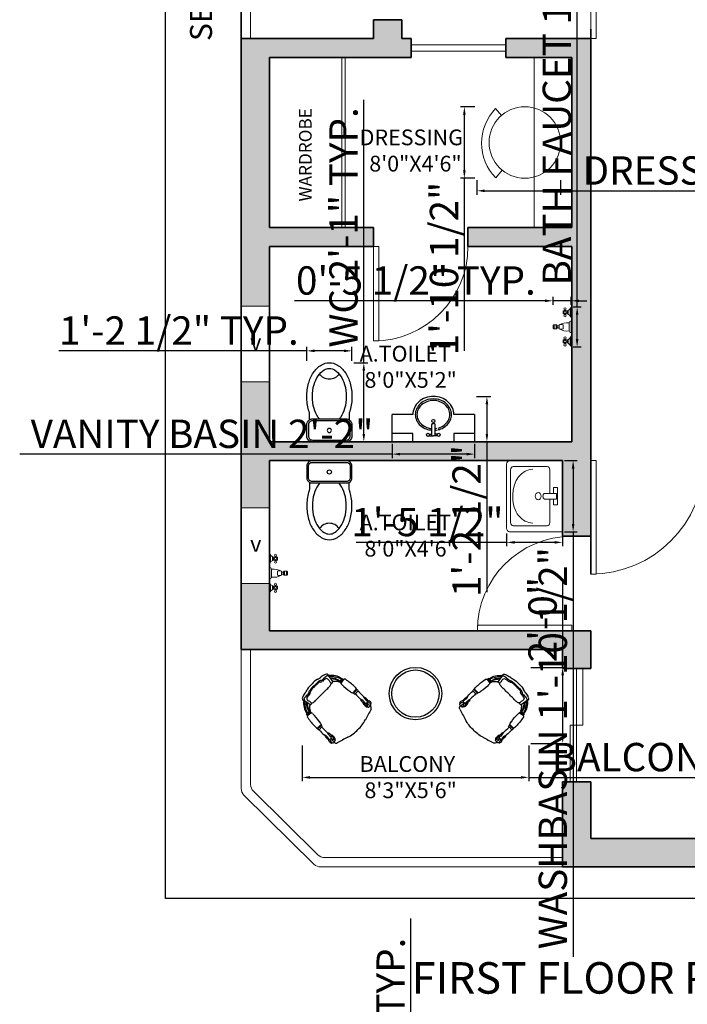
# Model space of a CAD drawing. Units: inches. Extents: x 3488 to 4319, y 780 to 1756.
# Tile 6 of 8: x 3844 to 4055, y 1274 to 1587. Entities that reach past the tile are written whole.
import ezdxf

# ---------------------------------------------------------------- set-up
doc = ezdxf.new("R2010")
doc.units = ezdxf.units.IN
for name, color, linetype, lineweight in [('A-ANNO-IDEN', 7, 'Continuous', 13), ('A-ANNO-TEXT', 7, 'Continuous', 18), ('A-ANNO-TITL', 7, 'Continuous', 25), ('A-AREA-IDEN', 7, 'Continuous', 18), ('A-DOOR', 4, 'Continuous', 18), ('A-FLOR-CASE', 32, 'Continuous', 18), ('A-FLOR-RAIL', 7, 'Continuous', 20), ('A-WALL', 7, 'Continuous', 35), ('A-WALL-PATT', 252, 'Continuous', 13), ('C-PROP', 7, 'Continuous', 25), ('DIM', 9, 'Continuous', 18), ('FUR', 42, 'Continuous', 18), ('window', 130, 'Continuous', 18), ('Сантехника', 9, 'Continuous', 18)]:
    doc.layers.add(name, color=color, linetype=linetype, lineweight=lineweight)
doc.layers.add('furn', color=7, linetype='Continuous')
doc.layers.add('SANTEH', color=7, linetype='Continuous')
doc.styles.get("Standard").update_dxf_attribs({"font": 'arial.ttf'})
doc.dimstyles.new('ISO-25', dxfattribs={"dimtxt": 9, "dimasz": 2.5, "dimexe": 1.25, "dimexo": 0.625, "dimtad": 1, "dimdec": 1, "dimlunit": 3, "dimtxsty": 'Standard', "dimcen": 2.5, "dimclrd": 1, "dimclre": 1, "dimclrt": 1, "dimadec": 0, "dimazin": 0, "dimtfac": 1, "dimtdec": 1, "dimtmove": 0, "dimatfit": 3, "dimfxl": 1, "dimarcsym": 0})

# ---------------------------------------------------------------- blocks, each defined once
blk = doc.blocks.new('*U3')
for p, q in [((0, 0), (0, -6)), ((36, 0), (36, -6))]:
    blk.add_line(p, q)
blk.add_lwpolyline([(0, 0), (0, 36), (1.75, 36), (1.75, 0)], close=True)
blk.add_arc((0, 0), 36, 0, 90)
blk = doc.blocks.new('*U9')
for p, q in [((0, 0), (0, 6)), ((36, 0), (36, 6))]:
    blk.add_line(p, q)
blk.add_lwpolyline([(0, 0), (0, -36), (1.75, -36), (1.75, 0)], close=True)
blk.add_arc((0, 0), 36, 270, 0)
blk = doc.blocks.new('*U10')
for p, q in [((0, 0), (0, 6)), ((30, 0), (30, 6))]:
    blk.add_line(p, q)
blk.add_lwpolyline([(0, 0), (0, -30), (1.75, -30), (1.75, 0)], close=True)
blk.add_arc((0, 0), 30, 270, 0)
blk = doc.blocks.new('*U11')
for p, q in [((-30, 0), (-30, 6)), ((0, 0), (0, 6))]:
    blk.add_line(p, q)
blk.add_lwpolyline([(0, 0), (0, -30), (-1.75, -30), (-1.75, 0)], close=True)
blk.add_arc((0, 0), 30, 180, 270)
blk = doc.blocks.new('K10-44')
at = {"layer": 'SANTEH'}
for points in [[(-182, 222.6, 0.020439), (-174, 197.6), (-174, 134.8, 0.262987), (-198.2, 92), (-198.2, -8, 0.414214), (-148.2, -58), (151.8, -58, 0.414214), (201.8, -8), (201.8, 92, 0.262987), (177.6, 134.8), (177.6, 197.6, 0.020439), (185.6, 222.6, 0.067459), (201.8, 342, 0.067459), (185.6, 461.3, 0.079812), (143.2, 554.1, 0.107118), (73.7, 621.5, 0.139889), (1.8, 642, 0.139889), (-70.1, 621.5, 0.107118), (-139.6, 554.1, 0.079812), (-182, 461.3, 0.067459), (-198.2, 342, 0.067459)], [(-148.2, 127), (151.8, 127, -0.414214), (186.8, 92), (186.8, -8, -0.414214), (151.8, -43), (-148.2, -43, -0.414214), (-183.2, -8), (-183.2, 92, -0.414214)]]:
    blk.add_lwpolyline(points, format="xyb", close=True, dxfattribs=at)
for points in [[(89.9, 142, 0.027307), (101.6, 157.6, 0.079812), (137.4, 235.9, 0.067459), (151.8, 342, 0.067459), (137.4, 448, 0.079812), (101.6, 526.4, 0.107118), (47.3, 579, 0.139889), (1.8, 592, 0.139889), (-43.7, 579, 0.107118), (-98, 526.4, 0.079812), (-133.8, 448, 0.067459), (-148.2, 342, 0.067459), (-133.8, 235.9, 0.079812), (-98, 157.6, 0.027307), (-86.4, 142, 0.139889)], [(-174, 134.8, -0.136371), (-148.2, 142), (151.8, 142, -0.136371), (177.6, 134.8)]]:
    blk.add_lwpolyline(points, format="xyb", dxfattribs=at)
blk.add_circle((1.8, 42), 18.3, dxfattribs=at)
blk.add_arc((1.8, 601.6), 105.3, 213.89944, 326.10056, dxfattribs=at)
blk = doc.blocks.new('s_20')
at = {"layer": 'SANTEH'}
for p, q in [((-1000, 0), (0, 0)), ((-1000, -330), (-1000, 0)), ((-750, -19), (-750, 0)), ((-250, 0), (-250, -100)), ((0, 0), (0, -330)), ((-1000, -100), (-750, -100)), ((-750, -100), (-750, -25)), ((-549, -73), (-500, -73)), ((-549, -93), (-520, -93)), ((-520, -73), (-520, -210)), ((-451, -73), (-500, -73)), ((-480, -73), (-480, -105)), ((-451, -93), (-480, -93)), ((-480, -109), (-480, -210)), ((-250, -100), (-35, -100)), ((-31, -100), (0, -100)), ((-510, -220), (-500, -220)), ((-490, -220), (-500, -220)), ((-1000, -330), (-750, -330)), ((-250, -330), (0, -330))]:
    blk.add_line(p, q, dxfattribs=at)
for points in [[(-720, -330, 0.110429), (-704, -400, 0.102661), (-657, -463, 0.093298), (-587, -505, 0.087608), (-500, -520, 0.087608), (-413, -505, 0.093298), (-343, -463, 0.102661), (-296, -400, 0.110429), (-280, -330, 0.110429), (-296, -260, 0.102661), (-343, -197, 0.093298), (-413, -155, 0.067743), (-480, -141, 0.087608)], [(-559, -147, 0.02908), (-587, -155, 0.093298), (-657, -197, 0.102661), (-704, -260, 0.110429), (-720, -330, 0.110429)], [(-700, -330, 0.110429), (-686, -391, 0.102661), (-644, -448, 0.093298), (-580, -486, 0.087608), (-500, -500, 0.087608), (-420, -486, 0.093298), (-356, -448, 0.102661), (-314, -391, 0.110429), (-300, -330, 0.110429), (-314, -269, 0.102661), (-356, -212, 0.093298), (-420, -174, 0.06604), (-480, -161, 0.087608)], [(-557, -167, 0.02562), (-580, -174, 0.093298), (-644, -212, 0.102661), (-686, -269, 0.110429), (-700, -330, 0.110429)], [(-520, -141, 0.028703), (-549, -145, 0.093298)], [(-520, -161, 0.024746), (-543, -164, 0.093298)], [(-750, -330, 0.110429), (-731, -413, 0.102661), (-677, -486, 0.093298), (-597, -533, 0.087608), (-500, -550, 0.087608), (-403, -533, 0.093298), (-323, -486, 0.102661), (-269, -413, 0.110429), (-250, -330, 0.110429)]]:
    blk.add_lwpolyline(points, format="xyb", dxfattribs=at)
for centre in [(-565, -84), (-435, -84), (-500, -252)]:
    blk.add_circle(centre, 18.9, dxfattribs=at)
for centre, start, end in [((-510, -210), 180, 270), ((-490, -210), 270, 0)]:
    blk.add_arc(centre, 10, start, end, dxfattribs=at)
blk = doc.blocks.new('Rac7')
at = {"color": 0}
for p, q in [((-39500.6, -24232.1), (-39500.6, -23829.6)), ((-39473.6, -23808.4), (-38988.3, -23808.4)), ((-39032.4, -23838), (-39429.6, -23838)), ((-38961.3, -23829.6), (-38961.3, -24232.1)), ((-39456.5, -23859.1), (-39456.5, -24114.9)), ((-39221.1, -23854.9), (-39240.8, -23854.9)), ((-39005.4, -24114.9), (-39005.4, -23859.1)), ((-39005.4, -23859.1), (-39005.4, -23859.1)), ((-39429.6, -24136.1), (-39252.5, -24136.1)), ((-39252.5, -24185.9), (-39252.5, -24093.6)), ((-39209.4, -24185.9), (-39209.4, -24093.6)), ((-39209.4, -24136.1), (-39032.4, -24136.1)), ((-39297, -24164), (-39252.5, -24164)), ((-39297, -24193.5), (-39297, -24164)), ((-39164.9, -24193.5), (-39297, -24193.5)), ((-39252.5, -24185.9), (-39209.4, -24185.9)), ((-39209.4, -24164), (-39164.9, -24164)), ((-39164.9, -24164), (-39164.9, -24193.5)), ((-38961.3, -24232.1), (-39500.6, -24232.1))]:
    blk.add_line(p, q, dxfattribs=at)
at = {"color": 0, "extrusion": (0, 0, -1)}
for centre, major_axis, start_param, end_param in [((-39473.6, -23829.6), (-27, 0), 0, 1.570796), ((-39429.6, -23859.1), (-27, 0), 0, 1.570796), ((-39032.4, -23859.1), (-27, 0), 1.570796, 3.141593), ((-38988.3, -23829.6), (-27, 0), 1.570796, 3.141593), ((-39240.8, -24007.4), (-194.1, 0), 0, 1.570796), ((-39221.1, -24007.4), (-194.1, 0), 1.570796, 3.141593), ((-39429.6, -24114.9), (-27, 0), -1.570796, 0), ((-39231, -24104), (-25.3, 0), 0.552816, 2.588777), ((-39032.4, -24114.9), (-27, 0), -3.141593, -1.570796)]:
    blk.add_ellipse(centre, major_axis=major_axis, ratio=0.785714, start_param=start_param, end_param=end_param, dxfattribs=at)
blk.add_ellipse((-39231, -24048), major_axis=(-27.9, 0), ratio=0.785714, dxfattribs=at)
blk = doc.blocks.new('Faucet - Bathroom front')
for p, q in [((-0.5, 4.25), (0.5, 4.25)), ((0.5, 3.75), (-0.5, 3.75)), ((-0.5, 3), (0.5, 3)), ((-0.25, 3), (-0.25, 3.5)), ((0.25, 3.5), (0.25, 3)), ((-5, 0), (-2.25, 0)), ((-4.5087, 0.25), (-2.7408, 0.25)), ((-4, 1.625), (-4.25, 1.625)), ((-4, 1.375), (-4.25, 1.375)), ((-3.1442, 0.75), (-4.0979, 0.75)), ((-3.25, 1.625), (-3, 1.625)), ((-3.25, 1.375), (-3, 1.375)), ((-1.5, 0), (1.5, 0)), ((-1, 0.5), (1, 0.5)), ((0.5, 2), (-0.5, 2)), ((2.25, 0), (5, 0)), ((2.7413, 0.25), (4.5092, 0.25)), ((3.25, 1.625), (3, 1.625)), ((3.25, 1.375), (3, 1.375)), ((4.1058, 0.75), (3.1521, 0.75)), ((4, 1.625), (4.25, 1.625)), ((4, 1.375), (4.25, 1.375))]:
    blk.add_line(p, q)
for points in [[(-0.5, 3.75), (-0.5, 4.25)], [(-0.25, 4.5), (0.25, 4.5)], [(0.25, 3.5), (-0.25, 3.5)], [(0.5, 4.25), (0.5, 3.75)]]:
    blk.add_lwpolyline(points)
for points in [[(-4, 1), (-4, 2), (-3.25, 2), (-3.25, 1)], [(3.25, 1), (3.25, 2), (4, 2), (4, 1)]]:
    blk.add_lwpolyline(points, close=True)
for centre in [(-4.5, 1.5), (-3.625, 1.5), (-2.75, 1.5), (2.75, 1.5), (3.625, 1.5), (4.5, 1.5)]:
    blk.add_circle(centre, 0.2795)
for centre, radius, start, end in [((3, 1), 4.0311, 150.2551, 187.125), ((0.6413, 2.5), 1.246, 156.3417, 203.6583), ((-0.2575, 4.2575), 0.2426, 88.22243, 181.7776), ((-0.2575, 3.7425), 0.2426, 178.2224, 271.7776), ((0.2575, 4.2575), 0.2426, 358.2224, 91.77757), ((0.2575, 3.7425), 0.2426, 268.2224, 1.777565), ((-3, 1), 4.0311, 352.875, 29.74488), ((-0.6413, 2.5), 1.246, 336.3417, 23.65835), ((-5.375, 1.375), 1.4252, 285.2551, 344.7449), ((-1.875, 1.375), 1.4252, 195.2551, 254.7449), ((-0.7962, -0.2038), 0.7327, 106.1502, 163.8498), ((0.7962, -0.2038), 0.7327, 16.1502, 73.84979), ((1.875, 1.375), 1.4252, 285.2551, 344.7449), ((5.375, 1.375), 1.4252, 195.2551, 254.7449)]:
    blk.add_arc(centre, radius, start, end)
blk = doc.blocks.new('ghean')
for p, q in [((36.9, 31.7), (0, 0)), ((331.1, 34.8), (373.2, 0.4))]:
    blk.add_line(p, q)
blk.add_circle((182.7, 156.7), 192)
blk.add_arc((186.4, 192.3), 267.8, 225.898, 314.2259)
blk = doc.blocks.new('CHAIR6')
at = {"layer": 'furn'}
for p, q in [((0.41, 0.26), (0.409, 0.318)), ((0.428, 0.318), (0.427, 0.263)), ((0.41, -0.26), (0.409, -0.318)), ((0.428, -0.318), (0.427, -0.263))]:
    blk.add_line(p, q, dxfattribs=at)
for centre in [(0.217, 0.287), (0.219, 0.277), (0.22, 0.268), (0.221, 0.26), (0.222, 0.252), (0.223, 0.243), (0.405, 0.315), (0.405, 0.306), (0.405, 0.298), (0.405, 0.29), (0.406, 0.281), (0.405, 0.273), (0.406, 0.264), (0.217, -0.287), (0.219, -0.277), (0.22, -0.268), (0.221, -0.26), (0.222, -0.252), (0.223, -0.243), (0.406, -0.264), (0.405, -0.273), (0.406, -0.281), (0.405, -0.29), (0.405, -0.298), (0.405, -0.306), (0.405, -0.315)]:
    blk.add_circle(centre, 0.00425, dxfattribs=at)
for centre, radius, start, end in [((0.231, 0.078), 0.206, 99.5359, 142.9697), ((0.288, -0.009), 0.296, 107.467, 135.6907), ((0.22, 0.084), 0.164, 95.986, 137.8084), ((0.297, -0.027), 0.289, 108.9658, 130.7483), ((0.27, 0.102), 0.148, 115.7424, 145.5422), ((0.2, 0.33), 0.0425, 267.3788, 299.5385), ((0.508, 0.309), 0.31, 183.9213, 193.664), ((0.217, 0.209), 0.0298, 85.8824, 112.3894), ((0.91, 0.35), 0.7, 184.9582, 189.1744), ((0.204, 0.356), 0.119, 277.5474, 281.9349), ((0.237, 0.291), 0.0162, 83.9773, 174.0092), ((2.236, 0.546), 2.032, 187.1641, 188.6742), ((0.243, 0.265), 0.029, 238.5377, 274.9353), ((0.372, -0.317), 0.638, 90.6066, 102.0554), ((0.251, 0.88), 0.644, 269.5737, 280.2481), ((0.377, 0.168), 0.153, 77.8964, 94.5268), ((0.357, 0.351), 0.106, 274.4213, 300.1481), ((3.364, 0.315), 2.963, 179.9011, 181.1479), ((0.418, 0.279), 0.04, 75.217, 102.1825), ((0.412, 0.301), 0.0413, 267.6069, 291.9537), ((0.471, 1.044), 0.775, 266.7794, 273.3084), ((0.481, -0.309), 0.624, 87.1388, 94.8424), ((0.516, 0.348), 0.0344, 262.5365, 295.1239), ((0.554, 0.405), 0.1, 244.9615, 286.9262), ((0.558, 0.149), 0.128, 78.3216, 109.437), ((0.517, 0.26), 0.0105, 7.9295, 98.404), ((0.548, 0.417), 0.157, 262.6911, 279.4279), ((0.557, 0.199), 0.121, 80.5687, 102.5802), ((0.576, 0.259), 0.00554, 151.0446, 320.6391), ((0.573, 0.254), 0.00119, 58.8883, 217.8317), ((0.586, 0.299), 0.0481, 252.1536, 277.044), ((0.575, 0.272), 0.00992, 261.0604, 17.0352), ((0.569, 0.306), 0.0148, 11.9312, 56.7136), ((0.6, 0.611), 0.349, 266.3251, 275.7659), ((0.586, 0.259), 0.00592, 143.235, 315.8485), ((0.557, 0.368), 0.0592, 293.7073, 312.3115), ((0.581, 0.292), 0.0168, 1.9585, 81.7578), ((0.571, 0.299), 0.0282, 299.2631, 346.0553), ((0.54, 0.261), 0.0504, 352.1945, 0.4931), ((0.596, 0.265), 0.012, 240.9156, 292.3604), ((0.599, 0.223), 0.0286, 84.2359, 104.2257), ((0.621, 0.242), 0.0492, 62.0869, 124.0669), ((0.596, 0.232), 0.05, 38.3646, 93.2736), ((0.627, 0.253), 0.0606, 83.3314, 123.5905), ((0.615, 0.273), 0.0542, 72.7266, 108.7219), ((0.63, 0.259), 0.03, 175.2542, 190.1424), ((0.604, 0.261), 0.00773, 242.6807, 299.2264), ((0.605, 0.322), 0.0704, 267.2787, 279.3344), ((0.623, 0.26), 0.0167, 173.5024, 200.3975), ((0.61, 0.258), 0.0049, 236.8473, 330.7161), ((0.646, 0.262), 0.0322, 179.9162, 191.0366), ((0.618, 0.257), 0.00347, 207.2761, 12.1204), ((0.62, 0.264), 0.0117, 254.3857, 324.079), ((0.626, 0.265), 0.00881, 232.8615, 349.2883), ((0.71, 0.267), 0.0896, 182.9909, 185.7082), ((0.629, 0.318), 0.00734, 318.7265, 73.2046), ((0.633, 0.295), 0.0177, 352.6874, 85.2992), ((0.635, 0.276), 0.0126, 270.9628, 46.1593), ((0.624, 0.308), 0.0303, 309.8512, 329.8717), ((0.651, 0.258), 0.0349, 27.0208, 91.1191), ((5.591, 1.641), 5.096, 195.566, 197.1124), ((-0.099, 0.131), 0.116, 336.0762, 0.2883), ((0.175, 0.114), 0.159, 153.5859, 173.6765), ((0.057, 0.18), 0.0247, 65.1084, 167.8729), ((0.009, 0.12), 0.0432, 336.8405, 13.1255), ((0.208, 0.139), 0.158, 161.7945, 183.4813), ((0.076, 0.176), 0.0215, 90.4966, 146.0411), ((0.234, 0.103), 0.171, 161.3786, 179.7853), ((0.075, 0.206), 0.00875, 210.7256, 277.1225), ((0.096, 0.134), 0.0336, 65.79, 135.3719), ((1.294, 7.349), 7.255, 260.3299, 260.9616), ((0.132, 0.233), 0.0718, 252.5123, 277.4747), ((0.142, 0.148), 0.0139, 39.5976, 92.786), ((0.101, 0.175), 0.0542, 340.1354, 9.9737), ((0.112, 0.126), 0.0505, 352.8157, 37.4708), ((-4.033, 0.095), 4.196, 358.7024, 0.3415), ((0.344, 0.019), 0.396, 357.2491, 18.1081), ((0.24, 0.022), 0.241, 165.2285, 185.2845), ((0.27, 0.033), 0.239, 166.6572, 187.8069), ((0.064, 0.08), 0.0277, 124.7421, 163.8327), ((0.458, 0.014), 0.416, 173.7493, 181.9752), ((0.09, 0.054), 0.0465, 139.2002, 173.5011), ((0.042, 0.101), 0.0209, 307.2671, 6.2804), ((0.24, -0.022), 0.241, 174.7155, 194.7715), ((-0.099, -0.131), 0.116, 359.7117, 23.9238), ((0.27, -0.033), 0.239, 172.1931, 193.3428), ((0.064, -0.08), 0.0277, 196.1673, 235.2579), ((0.458, -0.014), 0.416, 178.0248, 186.2507), ((0.09, -0.054), 0.0465, 186.4989, 220.7998), ((0.009, -0.12), 0.0432, 346.8745, 23.1595), ((0.042, -0.101), 0.0209, 353.7196, 52.7329), ((0.234, -0.103), 0.171, 180.2147, 198.6214), ((-4.033, -0.095), 4.196, 359.6585, 1.2976), ((0.344, -0.019), 0.396, 341.8919, 2.7509), ((0.175, -0.114), 0.159, 186.3235, 206.4141), ((0.057, -0.18), 0.0247, 192.1271, 294.8916), ((0.208, -0.139), 0.158, 176.5187, 198.2055), ((0.076, -0.176), 0.0215, 213.9589, 269.5034), ((0.075, -0.206), 0.00875, 82.8775, 149.2744), ((0.231, -0.078), 0.206, 217.0303, 260.4641), ((0.096, -0.134), 0.0336, 224.6281, 294.21), ((1.294, -7.349), 7.255, 99.0384, 99.6701), ((0.288, 0.009), 0.296, 224.3093, 252.533), ((0.22, -0.084), 0.164, 222.1916, 264.014), ((0.297, 0.027), 0.289, 229.2517, 251.0342), ((0.132, -0.233), 0.0718, 82.5253, 107.4877), ((0.142, -0.148), 0.0139, 267.214, 320.4024), ((0.27, -0.102), 0.148, 214.4578, 244.2576), ((0.112, -0.126), 0.0505, 322.5292, 7.1843), ((0.101, -0.175), 0.0542, 350.0263, 19.8646), ((5.591, -1.641), 5.096, 162.8876, 164.434), ((0.508, -0.309), 0.31, 166.336, 176.0787), ((0.2, -0.33), 0.0425, 60.4615, 92.6212), ((0.217, -0.209), 0.0298, 247.6106, 274.1176), ((0.91, -0.35), 0.7, 170.8256, 175.0418), ((0.204, -0.356), 0.119, 78.0651, 82.4526), ((2.236, -0.546), 2.032, 171.3258, 172.8359), ((0.237, -0.291), 0.0162, 185.9908, 276.0227), ((0.243, -0.265), 0.029, 85.0647, 121.4623), ((0.372, 0.317), 0.638, 257.9446, 269.3934), ((0.251, -0.88), 0.644, 79.7519, 90.4263), ((0.357, -0.351), 0.106, 59.8519, 85.5787), ((0.377, -0.168), 0.153, 265.4732, 282.1036), ((3.364, -0.315), 2.963, 178.8521, 180.0989), ((0.418, -0.279), 0.04, 257.8175, 284.783), ((0.412, -0.301), 0.0413, 68.0463, 92.3931), ((0.471, -1.044), 0.775, 86.6916, 93.2206), ((0.481, 0.309), 0.624, 265.1576, 272.8612), ((0.554, -0.405), 0.1, 73.0738, 115.0385), ((0.516, -0.348), 0.0344, 64.8761, 97.4635), ((0.517, -0.26), 0.0105, 261.596, 352.0705), ((0.558, -0.149), 0.128, 250.563, 281.6784), ((0.548, -0.417), 0.157, 80.5721, 97.3089), ((0.557, -0.199), 0.121, 257.4198, 279.4313), ((0.573, -0.254), 0.00119, 142.1683, 301.1117), ((0.576, -0.259), 0.00554, 39.3609, 208.9554), ((0.586, -0.299), 0.0481, 82.956, 107.8464), ((0.575, -0.272), 0.00992, 342.9648, 98.9396), ((0.569, -0.306), 0.0148, 303.2864, 348.0688), ((0.6, -0.611), 0.349, 84.2341, 93.6749), ((0.586, -0.259), 0.00592, 44.1515, 216.765), ((0.557, -0.368), 0.0592, 47.6885, 66.2927), ((0.581, -0.292), 0.0168, 278.2422, 358.0415), ((0.571, -0.299), 0.0282, 13.9447, 60.7369), ((0.596, -0.265), 0.012, 67.6396, 119.0844), ((0.54, -0.261), 0.0504, 359.5069, 7.8055), ((0.599, -0.223), 0.0286, 255.7743, 275.7641), ((0.596, -0.232), 0.05, 266.7264, 321.6354), ((0.621, -0.242), 0.0492, 235.9331, 297.9131), ((0.627, -0.253), 0.0606, 236.4095, 276.6686), ((0.615, -0.273), 0.0542, 251.2781, 287.2734), ((0.604, -0.261), 0.00773, 60.7736, 117.3193), ((0.63, -0.259), 0.03, 169.8576, 184.7458), ((0.605, -0.322), 0.0704, 80.6656, 92.7213), ((0.623, -0.26), 0.0167, 159.6025, 186.4976), ((0.61, -0.258), 0.0049, 29.2839, 123.1527), ((0.646, -0.262), 0.0322, 168.9634, 180.0838), ((0.618, -0.257), 0.00347, 347.8796, 152.7239), ((0.62, -0.264), 0.0117, 35.921, 105.6143), ((0.626, -0.265), 0.00881, 10.7117, 127.1385), ((0.71, -0.267), 0.0896, 174.2918, 177.0091), ((0.629, -0.318), 0.00734, 286.7954, 41.2735), ((0.633, -0.295), 0.0177, 274.7008, 7.3126), ((0.635, -0.276), 0.0126, 313.8407, 89.0372), ((0.624, -0.308), 0.0303, 30.1283, 50.1488), ((0.651, -0.258), 0.0349, 268.8809, 332.9792)]:
    blk.add_arc(centre, radius, start, end, dxfattribs=at)
blk = doc.blocks.new('A$C78847651')
at = {"layer": 'furn'}
for radius in [0.3, 0.27]:
    blk.add_circle((1.292, 0.566), radius, dxfattribs=at)
at = {"layer": 'furn', "rotation": 315}
blk.add_blockref('CHAIR6', (0.11, 0.677), dxfattribs=at)
at = {"layer": 'furn', "xscale": -1, "rotation": 44.99999999999991}
blk.add_blockref('CHAIR6', (2.474, 0.677), dxfattribs=at)
blk = doc.blocks.new('DOOR-SLIDING-36IN')
for p, q in [((2, 0), (2, 36)), ((4, 18), (4, 36)), ((0, 0), (0, 18)), ((0, 18), (4, 18))]:
    blk.add_line(p, q)
blk = doc.blocks.new('RAIL-BALCONY-CHAMFERED')
for p, q in [((0, 69), (0, 24.92)), ((3, 69), (3, 26.17)), ((23.12, 0.86), (0.89, 22.78)), ((24.35, 3.86), (3.89, 24.04)), ((102, 3), (26.46, 3)), ((102, 0), (25.23, 0))]:
    blk.add_line(p, q)
for centre, start, end in [((6, 26.17), 180, 225.4044), ((3, 24.92), 180, 225.4044), ((26.46, 6), 225.4044, 270), ((25.23, 3), 225.4044, 270)]:
    blk.add_arc(centre, 3, start, end)
blk = doc.blocks.new('DOOR-SLIDING-30IN')
for p, q in [((30, 2), (0, 2)), ((30, 0), (0, 0))]:
    blk.add_line(p, q)
blk = doc.blocks.new('*D58')
at = {"layer": 'Defpoints', "color": 0, "transparency": 16777216}
for p in [(3962.34, 1131.01), (3967.74, 1131.01), (3962.34, 1095.01)]:
    blk.add_point(p, dxfattribs=at)
at = {"layer": 'DIM', "color": 1, "lineweight": -2, "transparency": 16777216}
for p, q in [((3967.74, 1131.01), (3967.74, 1301.71)), ((3962.97, 1131.01), (3968.99, 1131.01)), ((3967.74, 1097.51), (3967.74, 1128.51)), ((3962.97, 1095.01), (3968.99, 1095.01))]:
    blk.add_line(p, q, dxfattribs=at)
at = {"layer": 'DIM', "color": 1, "transparency": 16777216}
for points in [[(3967.33, 1128.51), (3968.16, 1128.51), (3967.74, 1131.01)], [(3967.33, 1097.51), (3968.16, 1097.51), (3967.74, 1095.01)]]:
    blk.add_solid(points, dxfattribs=at)
at = {"layer": 'DIM', "color": 1, "transparency": 16777216, "insert": (3962.46, 1217.61), "char_height": 9, "attachment_point": 5, "rotation": 90}
blk.add_mtext('BALCONY SLIDER 3\'-0" TYP.', dxfattribs=at)
blk = doc.blocks.new('*D62')
at = {"layer": 'Defpoints', "color": 0, "transparency": 16777216}
for p in [(3949.01, 1478.16), (3952.78, 1478.16), (3949.01, 1453.07)]:
    blk.add_point(p, dxfattribs=at)
at = {"layer": 'DIM', "color": 1, "lineweight": -2, "transparency": 16777216}
for p, q in [((3952.78, 1478.16), (3952.78, 1561.58)), ((3949.64, 1478.16), (3954.03, 1478.16)), ((3952.78, 1455.57), (3952.78, 1475.66)), ((3949.64, 1453.07), (3954.03, 1453.07))]:
    blk.add_line(p, q, dxfattribs=at)
at = {"layer": 'DIM', "color": 1, "transparency": 16777216}
for points in [[(3952.36, 1475.66), (3953.19, 1475.66), (3952.78, 1478.16)], [(3952.36, 1455.57), (3953.19, 1455.57), (3952.78, 1453.07)]]:
    blk.add_solid(points, dxfattribs=at)
at = {"layer": 'DIM', "color": 1, "transparency": 16777216, "insert": (3947.5, 1521.12), "char_height": 9, "attachment_point": 5, "rotation": 90}
blk.add_mtext('WC 2\'-1" TYP.', dxfattribs=at)
blk = doc.blocks.new('*D63')
at = {"layer": 'Defpoints', "color": 0, "transparency": 16777216}
for p in [(3934.67, 1481.93), (3934.67, 1478.16), (3949.01, 1478.16)]:
    blk.add_point(p, dxfattribs=at)
at = {"layer": 'DIM', "color": 1, "lineweight": -2, "transparency": 16777216}
for p, q in [((3934.67, 1481.93), (3855.94, 1481.93)), ((3934.67, 1478.79), (3934.67, 1483.18)), ((3946.51, 1481.93), (3937.17, 1481.93)), ((3949.01, 1478.79), (3949.01, 1483.18))]:
    blk.add_line(p, q, dxfattribs=at)
at = {"layer": 'DIM', "color": 1, "transparency": 16777216}
for points in [[(3937.17, 1482.35), (3937.17, 1481.51), (3934.67, 1481.93)], [(3946.51, 1482.35), (3946.51, 1481.51), (3949.01, 1481.93)]]:
    blk.add_solid(points, dxfattribs=at)
at = {"layer": 'DIM', "color": 1, "transparency": 16777216, "insert": (3894.05, 1487.21), "char_height": 9, "attachment_point": 5}
blk.add_mtext('1\'-2 1/2" TYP.', dxfattribs=at)
blk = doc.blocks.new('*D64')
at = {"layer": 'Defpoints', "color": 0, "transparency": 16777216}
for p in [(4018.59, 1495.91), (4020.5, 1495.91), (4018.59, 1483.17)]:
    blk.add_point(p, dxfattribs=at)
at = {"layer": 'DIM', "color": 1, "lineweight": -2, "transparency": 16777216}
for p, q in [((4020.5, 1495.91), (4020.5, 1665.9)), ((4019.21, 1495.91), (4021.75, 1495.91)), ((4020.5, 1485.67), (4020.5, 1493.41)), ((4019.21, 1483.17), (4021.75, 1483.17))]:
    blk.add_line(p, q, dxfattribs=at)
at = {"layer": 'DIM', "color": 1, "transparency": 16777216}
for points in [[(4020.08, 1493.41), (4020.91, 1493.41), (4020.5, 1495.91)], [(4020.08, 1485.67), (4020.91, 1485.67), (4020.5, 1483.17)]]:
    blk.add_solid(points, dxfattribs=at)
at = {"layer": 'DIM', "color": 1, "transparency": 16777216, "insert": (4015.22, 1582.16), "char_height": 9, "attachment_point": 5, "rotation": 90}
blk.add_mtext('BATH FAUCET 1\'-0 1/2" TYP.', dxfattribs=at)
blk = doc.blocks.new('*D65')
at = {"layer": 'Defpoints', "color": 0, "transparency": 16777216}
for p in [(4012.85, 1497.82), (4012.85, 1495.91), (4018.59, 1495.91)]:
    blk.add_point(p, dxfattribs=at)
at = {"layer": 'DIM', "color": 1, "lineweight": -2, "transparency": 16777216}
for p, q in [((4010.35, 1497.82), (3930.77, 1497.82)), ((4012.85, 1496.54), (4012.85, 1499.07)), ((4018.59, 1497.82), (4012.85, 1497.82)), ((4018.59, 1496.54), (4018.59, 1499.07)), ((4021.09, 1497.82), (4023.59, 1497.82))]:
    blk.add_line(p, q, dxfattribs=at)
at = {"layer": 'DIM', "color": 1, "transparency": 16777216}
for points in [[(4010.35, 1498.24), (4010.35, 1497.41), (4012.85, 1497.82)], [(4021.09, 1498.24), (4021.09, 1497.41), (4018.59, 1497.82)]]:
    blk.add_solid(points, dxfattribs=at)
at = {"layer": 'DIM', "color": 1, "transparency": 16777216, "insert": (3969.31, 1503.1), "char_height": 9, "attachment_point": 5}
blk.add_mtext('0\'-5 1/2" TYP.', dxfattribs=at)
blk = doc.blocks.new('*D94')
at = {"layer": 'Defpoints', "color": 0, "transparency": 16777216}
for p in [(3961.8, 1453.07), (3987.94, 1453.07), (3961.8, 1449.15)]:
    blk.add_point(p, dxfattribs=at)
at = {"layer": 'DIM', "color": 1, "lineweight": -2, "transparency": 16777216}
for p, q in [((3961.8, 1452.44), (3961.8, 1447.9)), ((3987.94, 1452.44), (3987.94, 1447.9)), ((3961.8, 1449.15), (3843.53, 1449.15)), ((3985.44, 1449.15), (3964.3, 1449.15))]:
    blk.add_line(p, q, dxfattribs=at)
at = {"layer": 'DIM', "color": 1, "transparency": 16777216}
for points in [[(3964.3, 1449.56), (3964.3, 1448.73), (3961.8, 1449.15)], [(3985.44, 1449.56), (3985.44, 1448.73), (3987.94, 1449.15)]]:
    blk.add_solid(points, dxfattribs=at)
at = {"layer": 'DIM', "color": 1, "transparency": 16777216, "insert": (3901.42, 1454.42), "char_height": 9, "attachment_point": 5}
blk.add_mtext('VANITY BASIN 2\'-2"', dxfattribs=at)
blk = doc.blocks.new('*D95')
at = {"layer": 'Defpoints', "color": 0, "transparency": 16777216}
for p in [(3987.94, 1467.44), (3987.94, 1453.07), (3991.86, 1453.07)]:
    blk.add_point(p, dxfattribs=at)
at = {"layer": 'DIM', "color": 1, "lineweight": -2, "transparency": 16777216}
for p, q in [((3988.56, 1467.44), (3993.11, 1467.44)), ((3991.86, 1464.94), (3991.86, 1455.57)), ((3988.56, 1453.07), (3993.11, 1453.07)), ((3991.86, 1453.07), (3991.86, 1405.27))]:
    blk.add_line(p, q, dxfattribs=at)
at = {"layer": 'DIM', "color": 1, "transparency": 16777216}
for points in [[(3991.44, 1464.94), (3992.27, 1464.94), (3991.86, 1467.44)], [(3991.44, 1455.57), (3992.27, 1455.57), (3991.86, 1453.07)]]:
    blk.add_solid(points, dxfattribs=at)
at = {"layer": 'DIM', "color": 1, "transparency": 16777216, "insert": (3986.58, 1427.92), "char_height": 9, "attachment_point": 5, "rotation": 90}
blk.add_mtext('1\'-2 1/2"', dxfattribs=at)
blk = doc.blocks.new('*D96')
at = {"layer": 'Defpoints', "color": 0, "transparency": 16777216}
for p in [(4015.84, 1447.07), (4015.84, 1424.51), (4019.23, 1424.51)]:
    blk.add_point(p, dxfattribs=at)
at = {"layer": 'DIM', "color": 1, "lineweight": -2, "transparency": 16777216}
for p, q in [((4016.47, 1447.07), (4020.48, 1447.07)), ((4019.23, 1444.57), (4019.23, 1427.01)), ((4016.47, 1424.51), (4020.48, 1424.51)), ((4019.23, 1424.51), (4019.23, 1289.56))]:
    blk.add_line(p, q, dxfattribs=at)
at = {"layer": 'DIM', "color": 1, "transparency": 16777216}
for points in [[(4018.81, 1444.57), (4019.65, 1444.57), (4019.23, 1447.07)], [(4018.81, 1427.01), (4019.65, 1427.01), (4019.23, 1424.51)]]:
    blk.add_solid(points, dxfattribs=at)
at = {"layer": 'DIM', "color": 1, "transparency": 16777216, "insert": (4013.95, 1355.79), "char_height": 9, "attachment_point": 5, "rotation": 90}
blk.add_mtext('WASHBASIN 1\'-10 1/2"', dxfattribs=at)
blk = doc.blocks.new('*D97')
at = {"layer": 'Defpoints', "color": 0, "transparency": 16777216}
for p in [(3998.12, 1424.51), (4015.84, 1424.51), (3998.12, 1421.13)]:
    blk.add_point(p, dxfattribs=at)
at = {"layer": 'DIM', "color": 1, "lineweight": -2, "transparency": 16777216}
for p, q in [((3998.12, 1423.89), (3998.12, 1419.88)), ((4015.84, 1423.89), (4015.84, 1419.88)), ((3998.12, 1421.13), (3950.32, 1421.13)), ((4013.34, 1421.13), (4000.62, 1421.13))]:
    blk.add_line(p, q, dxfattribs=at)
at = {"layer": 'DIM', "color": 1, "transparency": 16777216}
for points in [[(4000.62, 1421.54), (4000.62, 1420.71), (3998.12, 1421.13)], [(4013.34, 1421.54), (4013.34, 1420.71), (4015.84, 1421.13)]]:
    blk.add_solid(points, dxfattribs=at)
at = {"layer": 'DIM', "color": 1, "transparency": 16777216, "insert": (3972.97, 1426.41), "char_height": 9, "attachment_point": 5}
blk.add_mtext('1\'-5 1/2"', dxfattribs=at)
blk = doc.blocks.new('*D98')
at = {"layer": 'Defpoints', "color": 0, "transparency": 16777216}
for p in [(3988.67, 1536.73), (4015.22, 1536.73), (4015.22, 1532.75)]:
    blk.add_point(p, dxfattribs=at)
at = {"layer": 'DIM', "color": 1, "lineweight": -2, "transparency": 16777216}
for p, q in [((3988.67, 1536.1), (3988.67, 1531.5)), ((4015.22, 1536.1), (4015.22, 1531.5)), ((3991.17, 1532.75), (4012.72, 1532.75)), ((4015.22, 1532.75), (4175.19, 1532.75))]:
    blk.add_line(p, q, dxfattribs=at)
at = {"layer": 'DIM', "color": 1, "transparency": 16777216}
for points in [[(3991.17, 1533.16), (3991.17, 1532.33), (3988.67, 1532.75)], [(4012.72, 1533.16), (4012.72, 1532.33), (4015.22, 1532.75)]]:
    blk.add_solid(points, dxfattribs=at)
at = {"layer": 'DIM', "color": 1, "transparency": 16777216, "insert": (4096.46, 1538.02), "char_height": 9, "attachment_point": 5}
blk.add_mtext('DRESSING CHAIR 2\'-2 1/2"', dxfattribs=at)
blk = doc.blocks.new('*D99')
at = {"layer": 'Defpoints', "color": 0, "transparency": 16777216}
for p in [(3988.67, 1559.41), (3984.69, 1536.73), (3988.67, 1536.73)]:
    blk.add_point(p, dxfattribs=at)
at = {"layer": 'DIM', "color": 1, "lineweight": -2, "transparency": 16777216}
for p, q in [((3988.05, 1559.41), (3983.44, 1559.41)), ((3984.69, 1556.91), (3984.69, 1539.23)), ((3988.05, 1536.73), (3983.44, 1536.73)), ((3984.69, 1536.73), (3984.69, 1481.94))]:
    blk.add_line(p, q, dxfattribs=at)
at = {"layer": 'DIM', "color": 1, "transparency": 16777216}
for points in [[(3984.28, 1556.91), (3985.11, 1556.91), (3984.69, 1559.41)], [(3984.28, 1539.23), (3985.11, 1539.23), (3984.69, 1536.73)]]:
    blk.add_solid(points, dxfattribs=at)
at = {"layer": 'DIM', "color": 1, "transparency": 16777216, "insert": (3979.41, 1508.08), "char_height": 9, "attachment_point": 5, "rotation": 90}
blk.add_mtext('1\'-10 1/2"', dxfattribs=at)
blk = doc.blocks.new('*D100')
at = {"layer": 'Defpoints', "color": 0, "transparency": 16777216}
for p in [(3933.23, 1357.29), (4005.13, 1357.29), (4005.13, 1346.51)]:
    blk.add_point(p, dxfattribs=at)
at = {"layer": 'DIM', "color": 1, "lineweight": -2, "transparency": 16777216}
for p, q in [((3933.23, 1356.67), (3933.23, 1345.26)), ((4005.13, 1356.67), (4005.13, 1345.26)), ((3935.73, 1346.51), (4002.63, 1346.51)), ((4005.13, 1346.51), (4154.67, 1346.51))]:
    blk.add_line(p, q, dxfattribs=at)
at = {"layer": 'DIM', "color": 1, "transparency": 16777216}
for points in [[(3935.73, 1346.93), (3935.73, 1346.09), (3933.23, 1346.51)], [(4002.63, 1346.93), (4002.63, 1346.09), (4005.13, 1346.51)]]:
    blk.add_solid(points, dxfattribs=at)
at = {"layer": 'DIM', "color": 1, "transparency": 16777216, "insert": (4081.15, 1351.79), "char_height": 9, "attachment_point": 5}
blk.add_mtext('BALCONY SEATING 6\'-0"', dxfattribs=at)
blk = doc.blocks.new('*D101')
at = {"layer": 'Defpoints', "color": 0, "transparency": 16777216}
for p in [(4005.13, 1381.44), (4015.91, 1381.44), (4005.13, 1357.29)]:
    blk.add_point(p, dxfattribs=at)
at = {"layer": 'DIM', "color": 1, "lineweight": -2, "transparency": 16777216}
for p, q in [((4015.91, 1381.44), (4015.91, 1409.27)), ((4005.75, 1381.44), (4017.16, 1381.44)), ((4015.91, 1359.79), (4015.91, 1378.94)), ((4005.75, 1357.29), (4017.16, 1357.29))]:
    blk.add_line(p, q, dxfattribs=at)
at = {"layer": 'DIM', "color": 1, "transparency": 16777216}
for points in [[(4015.49, 1378.94), (4016.33, 1378.94), (4015.91, 1381.44)], [(4015.49, 1359.79), (4016.33, 1359.79), (4015.91, 1357.29)]]:
    blk.add_solid(points, dxfattribs=at)
at = {"layer": 'DIM', "color": 1, "transparency": 16777216, "insert": (4010.69, 1396.61), "char_height": 9, "attachment_point": 5, "rotation": 90}
blk.add_mtext('2\'-0"', dxfattribs=at)

msp = doc.modelspace()

# ---------------------------------------------------------------- hatches: boundary and pattern name
at = {"layer": 'A-WALL-PATT', "transparency": 33554687}
h = msp.add_hatch(color=256, dxfattribs=at)
h.dxf.hatch_style = 1
h.paths.add_polyline_path([(4165.84, 1710.07), (3955.84, 1710.07), (3955.84, 1623.07), (3964.84, 1623.07), (3964.84, 1701.07), (4156.84, 1701.07), (4156.84, 1671.07), (4165.84, 1671.07)])
h.paths.add_polyline_path([(4165.84, 1611.07), (4156.84, 1611.07), (4156.84, 1581.07), (4060.84, 1581.07), (4060.84, 1575.07), (4156.84, 1575.07), (4156.84, 1569.1), (4165.84, 1569.1)])
h.paths.add_polyline_path([(3922.84, 1575.07), (3967.84, 1575.07), (3967.84, 1581.07), (3964.84, 1581.07), (3964.84, 1587.07), (3955.84, 1587.07), (3955.84, 1581.07), (3913.84, 1581.07), (3913.84, 1496.07), (3922.84, 1496.07), (3922.84, 1515.07), (3955.84, 1515.07), (3955.84, 1521.07), (3922.84, 1521.07)])
h.paths.add_polyline_path([(4024.84, 1575.07), (4024.84, 1581.07), (3997.84, 1581.07), (3997.84, 1575.07), (4018.84, 1575.07), (4018.84, 1521.07), (3985.84, 1521.07), (3985.84, 1515.07), (4018.84, 1515.07), (4018.84, 1453.07), (3922.84, 1453.07), (3922.84, 1472.07), (3913.84, 1472.07), (3913.84, 1432.07), (3922.84, 1432.07), (3922.84, 1447.07), (4015.84, 1447.07), (4015.84, 1424.51), (4015.84, 1423.07), (4024.84, 1423.07), (4024.84, 1447.07), (4024.84, 1453.07), (4024.84, 1503.07)])
h.paths.add_polyline_path([(3922.84, 1408.07), (3913.84, 1408.07), (3913.84, 1387.07), (4015.84, 1387.07), (4015.84, 1381.07), (4024.84, 1381.07), (4024.84, 1393.07), (4018.84, 1393.07), (3988.84, 1393.07), (3922.84, 1393.07)])
h.paths.add_polyline_path([(4165.84, 1459.04), (4156.84, 1459.04), (4156.84, 1453.07), (4060.84, 1453.07), (4060.84, 1447.07), (4156.84, 1447.07), (4156.84, 1327.07), (4151.87, 1327.07), (4137.84, 1327.07), (4137.84, 1318.07), (4165.84, 1318.07)])
h.paths.add_polyline_path([(4089.84, 1327.07), (4088.55, 1327.07), (4024.84, 1327.07), (4024.84, 1345.07), (4015.84, 1345.07), (4015.84, 1318.07), (4089.84, 1318.07)])
h.paths.add_polyline_path([(4165.84, 1545.1), (4156.84, 1545.1), (4156.84, 1483.04), (4165.84, 1483.04)])

# ---------------------------------------------------------------- linework, layer by layer
at = {"layer": 'A-FLOR-CASE'}
for p, q in [((3945.84, 1521.07), (3945.84, 1575.07)), ((3946.84, 1521.07), (3946.84, 1575.07)), ((4006.84, 1575.07), (4006.84, 1521.07))]:
    msp.add_line(p, q, dxfattribs=at)
at = {"layer": 'A-FLOR-RAIL'}
msp.add_line((3916.84, 1581.07), (3916.84, 1701.07), dxfattribs=at)
at = {"layer": 'A-WALL'}
for p, q in [((3913.84, 1387.07), (3913.84, 1710.07)), ((3955.84, 1587.07), (3964.84, 1587.07)), ((3955.84, 1587.07), (3955.84, 1581.07)), ((3964.84, 1587.07), (3964.84, 1581.07)), ((4024.84, 1575.07), (4024.84, 1584.07)), ((3913.84, 1581.07), (3955.84, 1581.07)), ((3964.84, 1581.07), (3967.84, 1581.07)), ((3967.84, 1581.07), (3967.84, 1575.07)), ((3997.84, 1581.07), (3997.84, 1575.07)), ((3997.84, 1581.07), (4024.84, 1581.07)), ((3922.84, 1575.07), (3967.84, 1575.07)), ((3922.84, 1521.07), (3922.84, 1575.07)), ((3997.84, 1575.07), (4018.84, 1575.07)), ((4018.84, 1575.07), (4018.84, 1521.07)), ((4024.84, 1575.07), (4024.84, 1447.07)), ((3922.84, 1521.07), (3955.84, 1521.07)), ((3955.84, 1521.07), (3955.84, 1515.07)), ((3985.84, 1521.07), (4018.84, 1521.07)), ((3985.84, 1521.07), (3985.84, 1515.07)), ((3922.84, 1515.07), (3955.84, 1515.07)), ((3922.84, 1453.07), (3922.84, 1515.07)), ((3985.84, 1515.07), (4018.84, 1515.07)), ((4018.84, 1515.07), (4018.84, 1453.07)), ((4024.84, 1503.07), (4024.84, 1411.07)), ((3922.84, 1453.07), (4018.84, 1453.07)), ((3922.84, 1393.07), (3922.84, 1447.07)), ((3922.84, 1447.07), (4015.84, 1447.07)), ((4015.84, 1447.07), (4015.84, 1423.07)), ((4015.84, 1423.07), (4024.84, 1423.07)), ((3922.84, 1393.07), (4024.84, 1393.07)), ((4024.84, 1393.07), (4024.84, 1381.07)), ((3913.84, 1387.07), (4015.84, 1387.07)), ((4015.84, 1387.07), (4015.84, 1381.07)), ((4015.84, 1381.07), (4024.84, 1381.07)), ((4015.84, 1345.07), (4024.84, 1345.07)), ((4015.84, 1345.07), (4015.84, 1318.07)), ((4024.84, 1345.07), (4024.84, 1327.07)), ((4024.84, 1327.07), (4156.84, 1327.07)), ((4015.84, 1318.07), (4165.84, 1318.07))]:
    msp.add_line(p, q, dxfattribs=at)
at = {"layer": 'C-PROP'}
for p, q in [((3889.84, 1308.07), (3889.84, 1728.07)), ((4189.84, 1308.07), (3889.84, 1308.07))]:
    msp.add_line(p, q, dxfattribs=at)
at = {"layer": 'window'}
for p, q in [((3922.84, 1496.07), (3913.84, 1496.07)), ((3922.84, 1472.07), (3913.84, 1472.07)), ((3922.84, 1432.07), (3913.84, 1432.07)), ((3922.84, 1408.07), (3913.84, 1408.07))]:
    msp.add_line(p, q, dxfattribs=at)

# ---------------------------------------------------------------- block references
at = {"layer": 'A-DOOR'}
for name, p in [('*U3', (4024.84, 1581.07)), ('DOOR-SLIDING-30IN', (3967.84, 1577.07)), ('*U10', (3955.84, 1515.07)), ('*U9', (4024.84, 1447.07)), ('DOOR-SLIDING-36IN', (4018.34, 1345.07))]:
    msp.add_blockref(name, p, dxfattribs=at)
at = {"layer": 'A-DOOR', "rotation": 270}
msp.add_blockref('*U11', (4018.84, 1393.07), dxfattribs=at)
at = {"layer": 'A-FLOR-RAIL'}
msp.add_blockref('RAIL-BALCONY-CHAMFERED', (3913.84, 1318.07), dxfattribs=at)
at = {"layer": 'FUR', "xscale": 0.05905515, "yscale": 0.05905515, "zscale": 0.05905515, "rotation": 270}
msp.add_blockref('ghean', (3994.63, 1558.86), dxfattribs=at)
at = {"layer": 'FUR', "xscale": 27.76712172265381, "yscale": 27.76712172265381, "zscale": 27.76712172265381}
msp.add_blockref('A$C78847651', (3933.29, 1357.4), dxfattribs=at)
at = {"layer": 'Сантехника'}
for name, p, xscale, yscale, zscale, rotation in [('Faucet - Bathroom front', (4018.59, 1489.54), 1.274234813154425, 1.274234813154425, 1.274234813154425, 90), ('s_20', (3961.8, 1453.07), 0.0261360463197561, 0.0261360463197561, 0.0261360463197561, 180), ('K10-44', (3941.9, 1444.99), 0.0358529150226637, 0.0358529150226637, 0.0358529150226637, 180), ('Rac7', (3002.23, -205.22), -0.0418294453001151, 0.0418294453001151, 0.0418294453001151, 90), ('Faucet - Bathroom front', (3922.84, 1411.34), -1.274234813154425, 1.274234813154425, 1.274234813154425, 270)]:
    msp.add_blockref(name, p, dxfattribs=dict(at, xscale=xscale, yscale=yscale, zscale=zscale, rotation=rotation))
at = {"layer": 'Сантехника', "xscale": -0.0358529150226637, "yscale": 0.0358529150226637, "zscale": 0.0358529150226637}
msp.add_blockref('K10-44', (3941.9, 1455.15), dxfattribs=at)

# ---------------------------------------------------------------- texts
at = {"layer": 'A-ANNO-IDEN'}
for p in [(3916.7, 1482.16), (3916.7, 1418.16)]:
    msp.add_text('v', height=5, dxfattribs=at).set_placement(p)
at = {"layer": 'A-ANNO-TEXT', "attachment_point": 1, "rotation": 90}
for s, insert, char_height in [('\\pxt7;{SETBACK-2\'0"}', (3897.59, 1580.28), 7), ('WARDROBE', (3932.22, 1529.35), 4)]:
    msp.add_mtext_dynamic_manual_height_columns(s, width=83.4163, gutter_width=25, heights=[0], dxfattribs=dict(at, insert=insert, char_height=char_height))
at = {"layer": 'A-ANNO-TITL', "insert": (3968.02, 1287.85), "char_height": 10, "attachment_point": 1}
msp.add_mtext_dynamic_manual_height_columns('FIRST FLOOR PLAN', width=202.5735, gutter_width=25, heights=[0], dxfattribs=at)
at = {"layer": 'A-AREA-IDEN', "char_height": 5, "attachment_point": 1}
for s, insert in [('DRESSING\\P  8\'0"X4\'6"', (3951.46, 1552.2)), ('A.TOILET\\P 8\'0"X5\'2"', (3951.46, 1483.53)), ('A.TOILET\\P 8\'0"X4\'6"', (3951.46, 1429.96)), ('BALCONY\\P 8\'3"X5\'6"', (3951.46, 1353.26))]:
    msp.add_mtext_dynamic_manual_height_columns(s, width=83.4163, gutter_width=25, heights=[0], dxfattribs=dict(at, insert=insert))

# ---------------------------------------------------------------- dimensions: what is measured, and where the dimension line sits
at = {"layer": 'DIM'}
for base, p1, p2, angle, text, picture, middle in [((4020.5, 1495.91), (4018.59, 1483.17), (4018.59, 1495.91), 90, 'BATH FAUCET <> TYP.', '*D64', (4015.22, 1582.16)), ((3952.78, 1478.16), (3949.01, 1453.07), (3949.01, 1478.16), 90, 'WC <> TYP.', '*D62', (3947.5, 1521.12)), ((4012.85, 1497.82), (4018.59, 1495.91), (4012.85, 1495.91), 180, '<> TYP.', '*D65', (3969.31, 1503.1)), ((3934.67, 1481.93), (3949.01, 1478.16), (3934.67, 1478.16), 180, '<> TYP.', '*D63', (3894.05, 1487.21)), ((3961.8, 1449.15), (3987.94, 1453.07), (3961.8, 1453.07), 180, 'VANITY BASIN <>', '*D94', (3901.42, 1454.42)), ((4019.23, 1424.51), (4015.84, 1447.07), (4015.84, 1424.51), 270, 'WASHBASIN <>', '*D96', (4013.95, 1355.79)), ((3967.74, 1131.01), (3962.34, 1095.01), (3962.34, 1131.01), 90, 'BALCONY SLIDER <> TYP.', '*D58', (3962.46, 1217.61))]:
    dim = msp.add_linear_dim(base=base, p1=p1, p2=p2, angle=angle, text=text, dimstyle='ISO-25', override={"dimdec": 1, "dimlfac": 1, "dimrnd": 0, "dimzin": 1, "dimdsep": 46, "dimlunit": 4, "dimfrac": 2}, dxfattribs=at)
    dim.commit()
    dim.dimension.update_dxf_attribs({"geometry": picture, "text_midpoint": middle})
for base, p1, p2, text, picture, middle in [((4015.2208, 1532.7463), (3988.6746, 1536.7283), (4015.2208, 1536.7283), 'DRESSING CHAIR <>', '*D98', (4096.4573, 1538.0248)), ((4005.13, 1346.51), (3933.23, 1357.29), (4005.13, 1357.29), 'BALCONY SEATING <>', '*D100', (4081.15, 1351.79))]:
    dim = msp.add_linear_dim(base=base, p1=p1, p2=p2, text=text, dimstyle='ISO-25', override={"dimdec": 1, "dimlfac": 1, "dimrnd": 0, "dimzin": 1, "dimdsep": 46, "dimlunit": 4, "dimfrac": 2}, dxfattribs=at)
    dim.commit()
    dim.dimension.update_dxf_attribs({"geometry": picture, "text_midpoint": middle})
for base, p1, p2, angle, picture, middle in [((3984.69, 1536.73), (3988.67, 1559.41), (3988.67, 1536.73), 270, '*D99', (3979.41, 1508.08)), ((3991.86, 1453.07), (3987.94, 1467.44), (3987.94, 1453.07), 270, '*D95', (3986.58, 1427.92)), ((3998.12, 1421.13), (4015.84, 1424.51), (3998.12, 1424.51), 180, '*D97', (3972.97, 1426.41)), ((4015.9113, 1381.4419), (4005.1265, 1357.2948), (4005.1265, 1381.4419), 90, '*D101', (4010.6912, 1396.6058))]:
    dim = msp.add_linear_dim(base=base, p1=p1, p2=p2, angle=angle, dimstyle='ISO-25', override={"dimdec": 1, "dimlfac": 1, "dimrnd": 0, "dimzin": 1, "dimdsep": 46, "dimlunit": 4, "dimfrac": 2}, dxfattribs=at)
    dim.commit()
    dim.dimension.update_dxf_attribs({"geometry": picture, "text_midpoint": middle})

doc.saveas('drawing.dxf')
